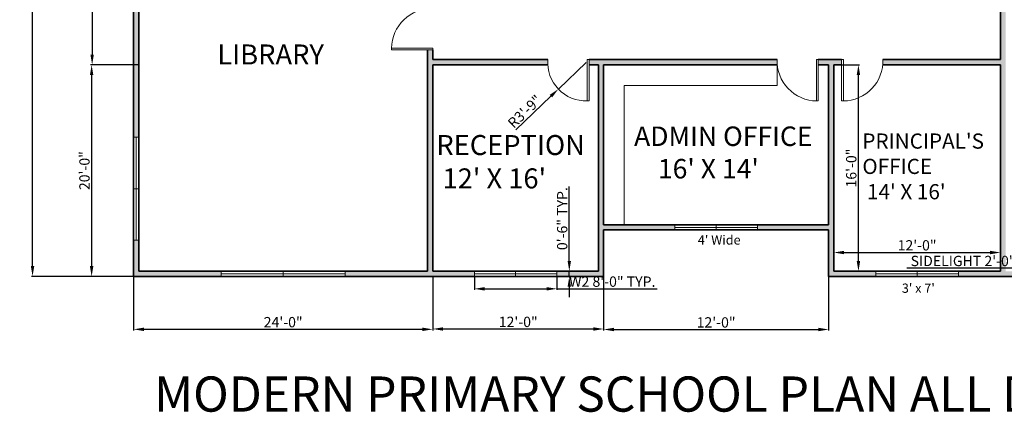
# Model space of a CAD drawing. Units: inches. Extents: x 2623 to 5095, y 1050 to 2384.
# Tile 1 of 4: x 2623 to 3768, y 1086 to 1542. Entities that reach past the tile are written whole.
import ezdxf

# ---------------------------------------------------------------- set-up
doc = ezdxf.new("R2010")
doc.units = ezdxf.units.IN
for name, color, linetype, lineweight in [('A-ANNO-DIMS', 2, 'Continuous', 13), ('A-ANNO-TEXT', 7, 'Continuous', 18), ('A-ANNO-TITL', 7, 'Continuous', 25), ('A-AREA-IDEN', 7, 'Continuous', 18), ('A-DOOR', 3, 'Continuous', 18), ('A-FLOR-CASE', 8, 'Continuous', 18), ('A-GLAZ', 4, 'Continuous', 18), ('A-WALL', 7, 'Continuous', 35)]:
    doc.layers.add(name, color=color, linetype=linetype, lineweight=lineweight)
doc.layers.add('A-WALL-PATT', color=251, linetype='Continuous', lineweight=9, true_color=0x636466)
doc.styles.get("Standard").update_dxf_attribs({"font": 'arial.ttf'})
doc.dimstyles.new('ISO-25', dxfattribs={"dimtxt": 12, "dimasz": 12, "dimexe": 1.25, "dimexo": 0.625, "dimtad": 1, "dimlunit": 3, "dimtxsty": 'Standard', "dimcen": 2.5, "dimadec": 0, "dimazin": 0, "dimtfac": 1, "dimtmove": 0, "dimatfit": 3, "dimfxl": 1, "dimarcsym": 0})

# ---------------------------------------------------------------- blocks, each defined once
blk = doc.blocks.new('*D11')
at = {"layer": 'A-ANNO-DIMS', "color": 0, "lineweight": -2, "transparency": 16777216}
for p, q in [((2761.1, 1729.6), (2706.4, 1729.6)), ((2707.6, 1717.6), (2707.6, 1501.6)), ((2761.1, 1489.6), (2706.4, 1489.6))]:
    blk.add_line(p, q, dxfattribs=at)
at = {"layer": 'A-ANNO-DIMS', "color": 0, "transparency": 16777216}
for points in [[(2705.6, 1717.6), (2709.6, 1717.6), (2707.6, 1729.6)], [(2705.6, 1501.6), (2709.6, 1501.6), (2707.6, 1489.6)]]:
    blk.add_solid(points, dxfattribs=at)
at = {"layer": 'Defpoints', "color": 0, "transparency": 16777216}
for p in [(2761.7, 1729.6), (2707.6, 1489.6), (2761.7, 1489.6)]:
    blk.add_point(p, dxfattribs=at)
at = {"layer": 'A-ANNO-DIMS', "color": 0, "transparency": 16777216, "insert": (2700.9, 1609.6), "char_height": 12, "attachment_point": 5, "rotation": 90}
blk.add_mtext('16\'-0"', dxfattribs=at)
blk = doc.blocks.new('*D12')
at = {"layer": 'A-ANNO-DIMS', "color": 0, "lineweight": -2, "transparency": 16777216}
for p, q in [((2755.1, 1489.6), (2705.7, 1489.6)), ((2707, 1477.6), (2707, 1255.6)), ((2755.1, 1243.6), (2705.7, 1243.6))]:
    blk.add_line(p, q, dxfattribs=at)
at = {"layer": 'A-ANNO-DIMS', "color": 0, "transparency": 16777216}
for points in [[(2705, 1477.6), (2709, 1477.6), (2707, 1489.6)], [(2705, 1255.6), (2709, 1255.6), (2707, 1243.6)]]:
    blk.add_solid(points, dxfattribs=at)
at = {"layer": 'Defpoints', "color": 0, "transparency": 16777216}
for p in [(2755.7, 1489.6), (2707, 1243.6), (2755.7, 1243.6)]:
    blk.add_point(p, dxfattribs=at)
at = {"layer": 'A-ANNO-DIMS', "color": 0, "transparency": 16777216, "insert": (2700.2, 1366.6), "char_height": 12, "attachment_point": 5, "rotation": 90}
blk.add_mtext('20\'-0"', dxfattribs=at)
blk = doc.blocks.new('*D13')
at = {"layer": 'A-ANNO-DIMS', "color": 0, "lineweight": -2, "transparency": 16777216}
for p, q in [((2755.7, 1243), (2755.7, 1180.9)), ((3103.7, 1243), (3103.7, 1180.9)), ((2767.7, 1182.1), (3091.7, 1182.1))]:
    blk.add_line(p, q, dxfattribs=at)
at = {"layer": 'A-ANNO-DIMS', "color": 0, "transparency": 16777216}
for points in [[(2767.7, 1184.1), (2767.7, 1180.1), (2755.7, 1182.1)], [(3091.7, 1184.1), (3091.7, 1180.1), (3103.7, 1182.1)]]:
    blk.add_solid(points, dxfattribs=at)
at = {"layer": 'Defpoints', "color": 0, "transparency": 16777216}
for p in [(2755.7, 1243.6), (3103.7, 1243.6), (3103.7, 1182.1)]:
    blk.add_point(p, dxfattribs=at)
at = {"layer": 'A-ANNO-DIMS', "color": 0, "transparency": 16777216, "insert": (2929.7, 1188.9), "char_height": 12, "attachment_point": 5}
blk.add_mtext('24\'-0"', dxfattribs=at)
blk = doc.blocks.new('*D14')
at = {"layer": 'A-ANNO-DIMS', "color": 0, "lineweight": -2, "transparency": 16777216}
for p, q in [((3103.7, 1243), (3103.7, 1181.2)), ((3302.3, 1243), (3302.3, 1181.2)), ((3115.7, 1182.5), (3290.3, 1182.5))]:
    blk.add_line(p, q, dxfattribs=at)
at = {"layer": 'A-ANNO-DIMS', "color": 0, "transparency": 16777216}
for points in [[(3115.7, 1184.5), (3115.7, 1180.5), (3103.7, 1182.5)], [(3290.3, 1184.5), (3290.3, 1180.5), (3302.3, 1182.5)]]:
    blk.add_solid(points, dxfattribs=at)
at = {"layer": 'Defpoints', "color": 0, "transparency": 16777216}
for p in [(3103.7, 1243.6), (3302.3, 1243.6), (3302.3, 1182.5)]:
    blk.add_point(p, dxfattribs=at)
at = {"layer": 'A-ANNO-DIMS', "color": 0, "transparency": 16777216, "insert": (3203, 1189.2), "char_height": 12, "attachment_point": 5}
blk.add_mtext('12\'-0"', dxfattribs=at)
blk = doc.blocks.new('*D15')
at = {"layer": 'A-ANNO-DIMS', "color": 0, "lineweight": -2, "transparency": 16777216}
for p, q in [((3302.3, 1243), (3302.3, 1180.6)), ((3563.9, 1243), (3563.9, 1180.6)), ((3314.3, 1181.9), (3551.9, 1181.9))]:
    blk.add_line(p, q, dxfattribs=at)
at = {"layer": 'A-ANNO-DIMS', "color": 0, "transparency": 16777216}
for points in [[(3314.3, 1183.9), (3314.3, 1179.9), (3302.3, 1181.9)], [(3551.9, 1183.9), (3551.9, 1179.9), (3563.9, 1181.9)]]:
    blk.add_solid(points, dxfattribs=at)
at = {"layer": 'Defpoints', "color": 0, "transparency": 16777216}
for p in [(3302.3, 1243.6), (3563.9, 1243.6), (3563.9, 1181.9)]:
    blk.add_point(p, dxfattribs=at)
at = {"layer": 'A-ANNO-DIMS', "color": 0, "transparency": 16777216, "insert": (3433.1, 1188.6), "char_height": 12, "attachment_point": 5}
blk.add_mtext('12\'-0"', dxfattribs=at)
blk = doc.blocks.new('*D25')
at = {"layer": 'A-ANNO-DIMS', "color": 0, "lineweight": -2, "transparency": 16777216}
for p, q in [((3570.5, 1489.6), (3599.8, 1489.6)), ((3598.6, 1261.6), (3598.6, 1477.6)), ((3570.5, 1249.6), (3599.8, 1249.6))]:
    blk.add_line(p, q, dxfattribs=at)
at = {"layer": 'A-ANNO-DIMS', "color": 0, "transparency": 16777216}
for points in [[(3596.6, 1477.6), (3600.6, 1477.6), (3598.6, 1489.6)], [(3596.6, 1261.6), (3600.6, 1261.6), (3598.6, 1249.6)]]:
    blk.add_solid(points, dxfattribs=at)
at = {"layer": 'Defpoints', "color": 0, "transparency": 16777216}
for p in [(3569.9, 1489.6), (3598.6, 1489.6), (3569.9, 1249.6)]:
    blk.add_point(p, dxfattribs=at)
at = {"layer": 'A-ANNO-DIMS', "color": 0, "transparency": 16777216, "insert": (3591.8, 1369.6), "char_height": 12, "attachment_point": 5, "rotation": 90}
blk.add_mtext('16\'-0"', dxfattribs=at)
blk = doc.blocks.new('*D26')
at = {"layer": 'A-ANNO-DIMS', "color": 0, "lineweight": -2, "transparency": 16777216}
for p, q in [((3569.9, 1250.2), (3569.9, 1272.7)), ((3581.9, 1271.4), (3751.7, 1271.4)), ((3763.7, 1250.2), (3763.7, 1272.7))]:
    blk.add_line(p, q, dxfattribs=at)
at = {"layer": 'A-ANNO-DIMS', "color": 0, "transparency": 16777216}
for points in [[(3581.9, 1273.4), (3581.9, 1269.4), (3569.9, 1271.4)], [(3751.7, 1273.4), (3751.7, 1269.4), (3763.7, 1271.4)]]:
    blk.add_solid(points, dxfattribs=at)
at = {"layer": 'Defpoints', "color": 0, "transparency": 16777216}
for p in [(3763.7, 1271.4), (3569.9, 1249.6), (3763.7, 1249.6)]:
    blk.add_point(p, dxfattribs=at)
at = {"layer": 'A-ANNO-DIMS', "color": 0, "transparency": 16777216, "insert": (3666.8, 1278.2), "char_height": 12, "attachment_point": 5}
blk.add_mtext('12\'-0"', dxfattribs=at)
blk = doc.blocks.new('WIN-144-DOUBLE-LIGHT')
for p, q in [((0, 6), (0, 0)), ((144, 3), (0, 3)), ((72, 6), (72, 0)), ((144, 6), (144, 0))]:
    blk.add_line(p, q)
blk = doc.blocks.new('WIN-96-DOUBLE-LIGHT')
for p, q in [((0, 6), (0, 0)), ((0, 3), (96, 3)), ((48, 6), (48, 0)), ((96, 6), (96, 0))]:
    blk.add_line(p, q)
blk = doc.blocks.new('WIN-120-DOUBLE-LIGHT')
for p, q in [((6, 120), (0, 120)), ((3, 120), (3, 0)), ((6, 60), (0, 60)), ((6, 0), (0, 0))]:
    blk.add_line(p, q)
blk = doc.blocks.new('DOOR-48-LEAF-AND-JAMBS')
for p, q in [((0, 48), (0, 0)), ((2, 48), (0, 48)), ((0, 48), (0, 42)), ((2, 0), (2, 48)), ((48, 48), (48, 42)), ((0, 0), (2, 0))]:
    blk.add_line(p, q)
blk = doc.blocks.new('*D53')
at = {"layer": 'A-ANNO-DIMS', "color": 0, "lineweight": -2, "transparency": 16777216}
for p, q in [((3152, 1243), (3152, 1228)), ((3248, 1243), (3248, 1228)), ((3164, 1229.2), (3236, 1229.2)), ((3248, 1229.2), (3364.7, 1229.2))]:
    blk.add_line(p, q, dxfattribs=at)
at = {"layer": 'A-ANNO-DIMS', "color": 0, "transparency": 16777216}
for points in [[(3164, 1231.2), (3164, 1227.2), (3152, 1229.2)], [(3236, 1231.2), (3236, 1227.2), (3248, 1229.2)]]:
    blk.add_solid(points, dxfattribs=at)
at = {"layer": 'Defpoints', "color": 0, "transparency": 16777216}
for p in [(3152, 1243.6), (3248, 1243.6), (3248, 1229.2)]:
    blk.add_point(p, dxfattribs=at)
at = {"layer": 'A-ANNO-DIMS', "color": 0, "transparency": 16777216, "insert": (3312.4, 1236), "char_height": 12, "attachment_point": 5}
blk.add_mtext('W2 8\'-0" TYP.', dxfattribs=at)
blk = doc.blocks.new('*D54')
at = {"layer": 'A-ANNO-DIMS', "color": 0, "lineweight": -2, "transparency": 16777216}
for p, q in [((3262.4, 1261.6), (3262.4, 1348)), ((3248.6, 1249.6), (3263.7, 1249.6)), ((3262.4, 1243.6), (3262.4, 1249.6)), ((3248.6, 1243.6), (3263.7, 1243.6)), ((3262.4, 1231.6), (3262.4, 1219.6))]:
    blk.add_line(p, q, dxfattribs=at)
at = {"layer": 'A-ANNO-DIMS', "color": 0, "transparency": 16777216}
for points in [[(3260.4, 1261.6), (3264.4, 1261.6), (3262.4, 1249.6)], [(3260.4, 1231.6), (3264.4, 1231.6), (3262.4, 1243.6)]]:
    blk.add_solid(points, dxfattribs=at)
at = {"layer": 'Defpoints', "color": 0, "transparency": 16777216}
for p in [(3248, 1249.6), (3262.4, 1249.6), (3248, 1243.6)]:
    blk.add_point(p, dxfattribs=at)
at = {"layer": 'A-ANNO-DIMS', "color": 0, "transparency": 16777216, "insert": (3255.7, 1310.8), "char_height": 12, "attachment_point": 5, "rotation": 90}
blk.add_mtext('0\'-6" TYP.', dxfattribs=at)
blk = doc.blocks.new('*D63')
at = {"layer": 'A-ANNO-DIMS', "color": 0, "lineweight": -2, "transparency": 16777216}
for p, q in [((3834.5, 1253.2), (3655, 1253.2)), ((3846.5, 1250.2), (3846.5, 1254.5)), ((3870.5, 1253.2), (3846.5, 1253.2)), ((3870.5, 1250.2), (3870.5, 1254.5)), ((3882.5, 1253.2), (3894.5, 1253.2))]:
    blk.add_line(p, q, dxfattribs=at)
at = {"layer": 'A-ANNO-DIMS', "color": 0, "transparency": 16777216}
for points in [[(3834.5, 1255.2), (3834.5, 1251.2), (3846.5, 1253.2)], [(3882.5, 1255.2), (3882.5, 1251.2), (3870.5, 1253.2)]]:
    blk.add_solid(points, dxfattribs=at)
at = {"layer": 'Defpoints', "color": 0, "transparency": 16777216}
for p in [(3846.5, 1253.2), (3846.5, 1249.6), (3870.5, 1249.6)]:
    blk.add_point(p, dxfattribs=at)
at = {"layer": 'A-ANNO-DIMS', "color": 0, "transparency": 16777216, "insert": (3738.8, 1260), "char_height": 12, "attachment_point": 5}
blk.add_mtext('SIDELIGHT 2\'-0" TYP.', dxfattribs=at)
blk = doc.blocks.new('*D66')
at = {"layer": 'A-ANNO-DIMS', "color": 0, "lineweight": -2, "transparency": 16777216}
for p, q in [((2755.1, 2251.6), (2637, 2251.6)), ((2638.3, 1255.6), (2638.3, 2239.6)), ((2755.1, 1243.6), (2637, 1243.6))]:
    blk.add_line(p, q, dxfattribs=at)
at = {"layer": 'A-ANNO-DIMS', "color": 0, "transparency": 16777216}
for points in [[(2636.3, 2239.6), (2640.3, 2239.6), (2638.3, 2251.6)], [(2636.3, 1255.6), (2640.3, 1255.6), (2638.3, 1243.6)]]:
    blk.add_solid(points, dxfattribs=at)
at = {"layer": 'Defpoints', "color": 0, "transparency": 16777216}
for p in [(2638.3, 2251.6), (2755.7, 2251.6), (2755.7, 1243.6)]:
    blk.add_point(p, dxfattribs=at)
at = {"layer": 'A-ANNO-DIMS', "color": 0, "transparency": 16777216, "insert": (2631.5, 1747.6), "char_height": 12, "attachment_point": 5, "rotation": 90}
blk.add_mtext('84\'-0"', dxfattribs=at)
blk = doc.blocks.new('*D74')
at = {"layer": 'A-ANNO-DIMS', "color": 0, "lineweight": -2, "transparency": 16777216}
for p, q in [((3282.1, 1492.4), (3249.7, 1461.4)), ((3200.1, 1413.9), (3241, 1453.1))]:
    blk.add_line(p, q, dxfattribs=at)
at = {"layer": 'A-ANNO-DIMS', "color": 0, "transparency": 16777216}
blk.add_solid([(3239.6, 1454.6), (3242.4, 1451.7), (3249.7, 1461.4)], dxfattribs=at)
at = {"layer": 'Defpoints', "color": 0, "transparency": 16777216}
for p in [(3282.1, 1492.4), (3249.7, 1461.4)]:
    blk.add_point(p, dxfattribs=at)
at = {"layer": 'A-ANNO-DIMS', "color": 0, "transparency": 16777216, "insert": (3211.6, 1434.2), "char_height": 12, "attachment_point": 5, "rotation": 43.7812}
blk.add_mtext('R3\'-9"', dxfattribs=at)

msp = doc.modelspace()

# ---------------------------------------------------------------- hatches: boundary and pattern name
at = {"layer": 'A-WALL-PATT'}
h = msp.add_hatch(color=256, dxfattribs=at)
h.dxf.hatch_style = 1
h.paths.add_polyline_path([(3103.717, 2251.615), (2755.717, 2251.615), (2755.717, 2173.615), (2761.717, 2173.615), (2761.717, 2245.615), (3097.717, 2245.615), (3097.717, 2015.688), (3100.811, 2015.688, -0.01561511), (3103.717, 2015.688)])
h.paths.add_polyline_path([(3103.717, 1967.688), (3097.717, 1967.688), (3097.717, 1957.615), (2761.717, 1957.615), (2761.717, 2029.615), (2755.717, 2029.615), (2755.717, 1915.615), (2761.717, 1915.615), (2761.717, 1951.615), (3097.717, 1951.615), (3097.717, 1943.747), (3103.717, 1943.747)])
h.paths.add_polyline_path([(3103.717, 1895.747, -0.01327118), (3101.235, 1895.747), (3097.717, 1895.747), (3097.717, 1735.615), (2761.717, 1735.615), (2761.717, 1771.615), (2755.717, 1771.615), (2755.717, 1693.615), (2761.717, 1693.615), (2761.717, 1729.615), (3097.717, 1729.615), (3097.717, 1721.81), (3103.717, 1721.81)])
h.paths.add_polyline_path([(2761.717, 1573.615), (2755.717, 1573.615), (2755.717, 1405.615), (2761.717, 1405.615)])
h.paths.add_polyline_path([(2761.717, 1285.615), (2755.717, 1285.615), (2755.717, 1243.615), (2857.717, 1243.615), (2857.717, 1249.615), (2761.717, 1249.615)])
h.paths.add_polyline_path([(3152.017, 1249.615), (3103.717, 1249.615), (3103.717, 1489.615), (3237.319, 1489.615, -0.03349431), (3237.344, 1495.615), (3103.717, 1495.615), (3103.717, 1507.046), (3097.717, 1507.046), (3097.717, 1249.615), (3001.717, 1249.615), (3001.717, 1243.615), (3103.717, 1243.615), (3152.017, 1243.615)])
h.paths.add_polyline_path([(3103.717, 1673.81, -0.01537929), (3100.853, 1673.81), (3097.717, 1673.81), (3097.717, 1555.046), (3101.163, 1555.046, -0.01366836), (3103.717, 1555.046)])
h.paths.add_polyline_path([(3302.317, 1249.615), (3302.317, 1297.615), (3385.117, 1297.615), (3385.117, 1303.615), (3302.317, 1303.615), (3302.317, 1489.615), (3503.954, 1489.615), (3503.954, 1492.911, -0.01449155), (3503.954, 1495.615), (3285.344, 1495.615), (3285.344, 1489.615), (3296.317, 1489.615), (3296.317, 1249.615), (3248.017, 1249.615), (3248.017, 1243.615), (3302.317, 1243.615)])
h.paths.add_polyline_path([(3569.917, 1489.615), (3579.094, 1489.615), (3579.094, 1495.615), (3551.954, 1495.615), (3551.954, 1489.615), (3563.917, 1489.615), (3563.917, 1303.615), (3481.117, 1303.615), (3481.117, 1297.615), (3563.917, 1297.615), (3563.917, 1249.615), (3563.917, 1243.615), (3618.817, 1243.615), (3618.817, 1249.615), (3569.917, 1249.615)])
h.paths.add_polyline_path([(3846.517, 1249.615), (3769.717, 1249.615), (3769.717, 1573.615), (3846.517, 1573.615), (3846.517, 1579.615), (3769.717, 1579.615), (3769.717, 1654.615), (3763.717, 1654.615), (3763.717, 1495.615), (3627.094, 1495.615, -0.01677945), (3627.094, 1492.499), (3627.094, 1489.615), (3763.717, 1489.615), (3763.717, 1249.615), (3714.817, 1249.615), (3714.817, 1243.615), (3763.717, 1243.615), (3846.517, 1243.615)])
h.paths.add_polyline_path([(4084.941, 1249.615), (4073.317, 1249.615), (4073.317, 1305.13), (4067.317, 1305.13), (4067.317, 1249.615), (3990.517, 1249.615), (3990.517, 1243.615), (4084.941, 1243.615)])
h.paths.add_polyline_path([(4277.411, 1249.615), (4208.317, 1249.615), (4208.317, 1366.615), (4282.724, 1366.615), (4282.724, 1370.675, -0.01031167), (4282.724, 1372.615), (4115.317, 1372.615), (4115.317, 1381.792), (4114.62, 1381.792, -0.02925374), (4109.317, 1381.792), (4109.317, 1372.615), (4073.317, 1372.615), (4067.317, 1372.615), (4067.317, 1353.13), (4073.317, 1353.13), (4073.317, 1366.615), (4202.317, 1366.615), (4202.317, 1249.615), (4120.941, 1249.615), (4120.941, 1243.615), (4277.411, 1243.615)])
h.paths.add_polyline_path([(4939.717, 1300.615), (4933.717, 1300.615), (4818.498, 1300.615), (4818.498, 1294.615), (4933.717, 1294.615), (4933.717, 1249.615), (4349.317, 1249.615), (4349.317, 1294.615), (4465.249, 1294.615), (4465.249, 1300.615), (4349.317, 1300.615), (4349.317, 1573.615), (4430.317, 1573.615), (4430.317, 1579.615), (4358.917, 1579.615), (4358.917, 1873.615), (4365.566, 1873.615), (4365.566, 1879.615), (4345.539, 1879.615), (4345.539, 1873.615), (4352.917, 1873.615), (4352.917, 1579.615), (4282.117, 1579.615), (4282.117, 1573.615), (4343.317, 1573.615), (4343.317, 1456.615), (4177.166, 1456.615), (4177.166, 1450.615), (4343.317, 1450.615), (4343.317, 1372.615), (4330.724, 1372.615), (4330.724, 1366.615), (4343.317, 1366.615), (4343.317, 1249.615), (4313.411, 1249.615), (4313.411, 1243.615), (4939.717, 1243.615)])

# ---------------------------------------------------------------- linework, layer by layer
at = {"layer": 'A-DOOR'}
for centre, radius, start, end in [((3102.44, 1508.335), 46.728, 88.433819, 179.12843), ((3282.065, 1492.431), 44.834, 175.927724, 271.634525), ((3550.587, 1494.263), 46.652, 178.339507, 269.222742), ((3580.676, 1494.057), 46.444, 270.515148, 1.922603)]:
    msp.add_arc(centre, radius, start, end, dxfattribs=at)
at = {"layer": 'A-FLOR-CASE'}
for p, q in [((3503.954, 1465.615), (3503.954, 1489.615)), ((3326.317, 1465.615), (3326.317, 1303.615)), ((3326.317, 1465.615), (3503.954, 1465.615))]:
    msp.add_line(p, q, dxfattribs=at)
at = {"layer": 'A-WALL'}
for p, q in [((2755.717, 1243.615), (2755.717, 2251.615)), ((3763.717, 1879.615), (3763.717, 1495.615)), ((2761.717, 1729.615), (2761.717, 1249.615)), ((3097.717, 1507.046), (3097.717, 1249.615)), ((3103.717, 1507.046), (3103.717, 1495.615)), ((3103.717, 1495.615), (3237.344, 1495.615)), ((3103.717, 1489.615), (3237.344, 1489.615)), ((3103.717, 1489.615), (3103.717, 1249.615)), ((3285.344, 1495.615), (3503.954, 1495.615)), ((3285.344, 1489.615), (3296.317, 1489.615)), ((3296.317, 1489.615), (3296.317, 1249.615)), ((3302.317, 1489.615), (3302.317, 1303.615)), ((3302.317, 1489.615), (3503.954, 1489.615)), ((3551.954, 1495.615), (3579.094, 1495.615)), ((3551.954, 1489.615), (3563.917, 1489.615)), ((3563.917, 1489.615), (3563.917, 1303.615)), ((3569.917, 1489.615), (3569.917, 1249.615)), ((3569.917, 1489.615), (3579.094, 1489.615)), ((3627.094, 1495.615), (3763.717, 1495.615)), ((3627.094, 1489.615), (3763.717, 1489.615)), ((3763.717, 1489.615), (3763.717, 1249.615)), ((3302.317, 1303.615), (3563.917, 1303.615)), ((3302.317, 1297.615), (3563.917, 1297.615)), ((3302.317, 1297.615), (3302.317, 1249.615)), ((3563.917, 1297.615), (3563.917, 1249.615)), ((3097.717, 1249.615), (2761.717, 1249.615)), ((3103.717, 1249.615), (3296.317, 1249.615)), ((3302.317, 1249.615), (3302.317, 1243.615)), ((3563.917, 1249.615), (3563.917, 1243.615)), ((3569.917, 1249.615), (3763.717, 1249.615)), ((3103.717, 1243.615), (2755.717, 1243.615)), ((3103.717, 1243.615), (3302.317, 1243.615)), ((3563.917, 1243.615), (3763.717, 1243.615)), ((3763.717, 1243.615), (3870.517, 1243.615))]:
    msp.add_line(p, q, dxfattribs=at)

# ---------------------------------------------------------------- block references
at = {"layer": 'A-DOOR', "extrusion": (0, 0, -1), "zscale": -1, "rotation": 90.00000000000345}
msp.add_blockref('DOOR-48-LEAF-AND-JAMBS', (-3055.717, 1507.046), dxfattribs=at)
at = {"layer": 'A-DOOR', "extrusion": (0, 0, -1), "zscale": -1}
for p in [(-3285.344, 1447.615), (-3551.954, 1447.615)]:
    msp.add_blockref('DOOR-48-LEAF-AND-JAMBS', p, dxfattribs=at)
at = {"layer": 'A-DOOR'}
msp.add_blockref('DOOR-48-LEAF-AND-JAMBS', (3579.094, 1447.615), dxfattribs=at)
at = {"layer": 'A-GLAZ'}
for name, p in [('WIN-120-DOUBLE-LIGHT', (2755.717, 1285.615)), ('WIN-96-DOUBLE-LIGHT', (3385.117, 1297.615)), ('WIN-144-DOUBLE-LIGHT', (2857.717, 1243.615)), ('WIN-96-DOUBLE-LIGHT', (3152.017, 1243.615)), ('WIN-96-DOUBLE-LIGHT', (3618.817, 1243.615))]:
    msp.add_blockref(name, p, dxfattribs=at)

# ---------------------------------------------------------------- texts
at = {"layer": 'A-ANNO-TEXT', "char_height": 10.7617, "attachment_point": 1}
for s, insert in [("4' Wide", (3411.878, 1291.401)), ("3' x 7'", (3649.076, 1235.328))]:
    msp.add_mtext_dynamic_manual_height_columns(s, width=391.78395, gutter_width=53.809, heights=[0], dxfattribs=dict(at, insert=insert))
at = {"layer": 'A-ANNO-TITL', "insert": (2779.618, 1127.325), "char_height": 40.95464, "attachment_point": 1}
msp.add_mtext_dynamic_manual_height_columns('MODERN PRIMARY SCHOOL PLAN ALL DIMENSIONS IN FEET', width=1853.61769, gutter_width=204.773, heights=[0], dxfattribs=at)
at = {"layer": 'A-AREA-IDEN', "attachment_point": 1}
for s, width, gutter_width, insert, char_height in [('LIBRARY', 847.02168, 116.332, (2853.229, 1513.256), 23.2665), ("RECEPTION\\P 12' X 16'", 847.02168, 116.332, (3107.85, 1407.977), 23.2665), ("ADMIN OFFICE\\P    16' X 14'", 824.72693, 113.27, (3337.72, 1417.896), 22.65406), ("PRINCIPAL'S\\POFFICE\\P 14' X 16'", 642.72757, 88.274, (3603.16, 1409.781), 17.6548)]:
    msp.add_mtext_dynamic_manual_height_columns(s, width=width, gutter_width=gutter_width, heights=[0], dxfattribs=dict(at, insert=insert, char_height=char_height))

# ---------------------------------------------------------------- dimensions: what is measured, and where the dimension line sits
at = {"layer": 'A-ANNO-DIMS'}
dim = msp.add_linear_dim(base=(2638.267, 2251.615), p1=(2755.717, 1243.615), p2=(2755.717, 2251.615), angle=90, dimstyle='ISO-25', override={"dimdec": 1, "dimlfac": 1, "dimrnd": 0, "dimzin": 1, "dimdsep": 46, "dimlunit": 4, "dimfrac": 2}, dxfattribs=at)
dim.commit()
dim.dimension.update_dxf_attribs({"geometry": '*D66', "text_midpoint": (2631.516, 1747.615)})
for base, p1, p2, angle, text, override, picture, middle in [((2707.618, 1489.615), (2761.717, 1729.615), (2761.717, 1489.615), 90, '16\'-0"', {"dimclrd": 0, "dimclre": 0, "dimclrt": 0}, '*D11', (2700.866, 1609.615)), ((2706.957, 1243.615), (2755.717, 1489.615), (2755.717, 1243.615), 90, '20\'-0"', {"dimclrd": 0, "dimclre": 0, "dimclrt": 0}, '*D12', (2700.205, 1366.615)), ((3598.595, 1489.615), (3569.917, 1249.615), (3569.917, 1489.615), 90, '16\'-0"', {"dimclrd": 0, "dimclre": 0, "dimclrt": 0}, '*D25', (3591.843, 1369.615)), ((3262.417, 1249.615), (3248.017, 1243.615), (3248.017, 1249.615), 90, '<> TYP.', {"dimdec": 1, "dimlfac": 1, "dimrnd": 0, "dimzin": 1, "dimdsep": 46, "dimlunit": 4, "dimfrac": 2}, '*D54', (3255.666, 1310.813)), ((3846.517, 1253.215), (3870.517, 1249.615), (3846.517, 1249.615), 180, 'SIDELIGHT <> TYP.', {"dimdec": 1, "dimlfac": 1, "dimrnd": 0, "dimzin": 1, "dimdsep": 46, "dimlunit": 4, "dimfrac": 2}, '*D63', (3738.772, 1260.045))]:
    dim = msp.add_linear_dim(base=base, p1=p1, p2=p2, angle=angle, text=text, dimstyle='ISO-25', override=override, dxfattribs=at)
    dim.commit()
    dim.dimension.update_dxf_attribs({"geometry": picture, "text_midpoint": middle})
dim = msp.add_radius_dim(center=(3282.065, 1492.431), mpoint=(3249.695, 1461.41), dimstyle='ISO-25', override={"dimdec": 1, "dimlfac": 1, "dimrnd": 0, "dimzin": 1, "dimdsep": 46, "dimlunit": 4, "dimfrac": 2}, dxfattribs=at)
dim.commit()
dim.dimension.update_dxf_attribs({"geometry": '*D74', "text_midpoint": (3211.58, 1434.241)})
for base, p1, p2, text, override, picture, middle in [((3763.717, 1271.412), (3569.917, 1249.615), (3763.717, 1249.615), '12\'-0"', {"dimclrd": 0, "dimclre": 0, "dimclrt": 0}, '*D26', (3666.817, 1278.164)), ((3248.017, 1229.215), (3152.017, 1243.615), (3248.017, 1243.615), 'W2 <> TYP.', {"dimdec": 1, "dimlfac": 1, "dimrnd": 0, "dimzin": 1, "dimdsep": 46, "dimlunit": 4, "dimfrac": 2}, '*D53', (3312.363, 1235.967)), ((3103.717, 1182.115), (2755.717, 1243.615), (3103.717, 1243.615), '24\'-0"', {"dimclrd": 0, "dimclre": 0, "dimclrt": 0}, '*D13', (2929.717, 1188.867)), ((3302.317, 1182.454), (3103.717, 1243.615), (3302.317, 1243.615), '12\'-0"', {"dimclrd": 0, "dimclre": 0, "dimclrt": 0}, '*D14', (3203.017, 1189.205)), ((3563.917, 1181.894), (3302.317, 1243.615), (3563.917, 1243.615), '12\'-0"', {"dimclrd": 0, "dimclre": 0, "dimclrt": 0}, '*D15', (3433.117, 1188.646))]:
    dim = msp.add_linear_dim(base=base, p1=p1, p2=p2, text=text, dimstyle='ISO-25', override=override, dxfattribs=at)
    dim.commit()
    dim.dimension.update_dxf_attribs({"geometry": picture, "text_midpoint": middle})

doc.saveas('drawing.dxf')
